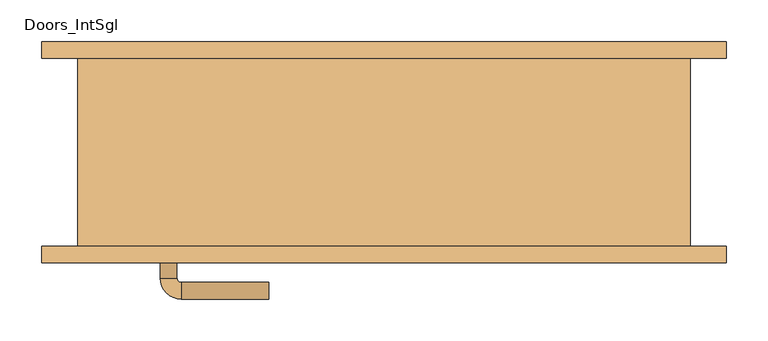
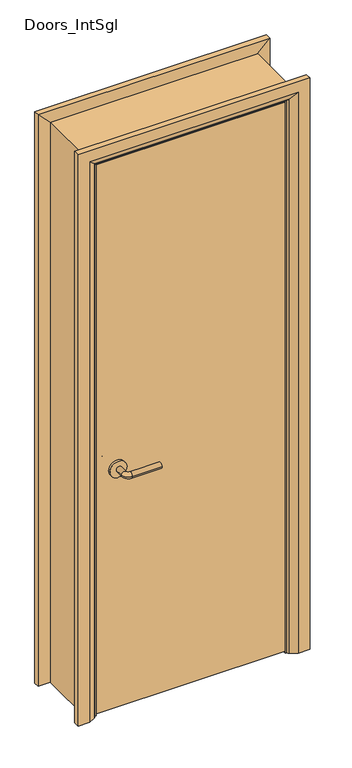
"""IFC4 building model written with IfcOpenShell, lengths in millimetres: door geometry, Doors_IntSgl."""

from ifc_helpers import new_model, si_unit, point, frame, frame_2d, origin, place, context, project, spatial, polyline, circle_curve, ellipse_curve, trimmed, segment, composite_curve, outline, extrude, faceted_brep, source, transform, mapped, element, save
from ifc_brep_helpers import plane_surface, cylinder_surface, revolved_surface, advanced_brep


def doors_intsgl_927b0b89(model_context):
    return source(origin(), model_context, "Body", "SolidModel", [
        advanced_brep(
        [(-268.0, -66.5, 900.0), (-248.0, -66.5, 900.0), (-268.0, -36.5, 900.0), (-248.0, -36.5, 900.0), (-243.0, -31.5, 900.0), (-243.0, -11.5, 900.0), (-138.0, -11.5, 900.0), (-138.0, -31.5, 900.0)],
        [
            (0, 1, circle_curve(frame((-258.0, -66.5, 900.0), z_axis=(0.0, -1.0, 0.0), x_axis=(1.0, 0.0, 0.0)), 10.0)),
            (1, 0, circle_curve(frame((-258.0, -66.5, 900.0), z_axis=(0.0, -1.0, 0.0), x_axis=(1.0, 0.0, 0.0)), 10.0)),
            (0, 2),
            (2, 3, circle_curve(frame((-258.0, -36.5, 900.0), z_axis=(0.0, -1.0, 0.0), x_axis=(1.0, 0.0, 0.0)), 10.0)),
            (3, 1),
            (3, 2, circle_curve(frame((-258.0, -36.5, 900.0), z_axis=(0.0, -1.0, 0.0), x_axis=(1.0, 0.0, 0.0)), 10.0)),
            (4, 3, circle_curve(frame((-243.0, -36.5, 900.0), z_axis=(0.0, 0.0, 1.0), x_axis=(-1.0, 0.0, 0.0)), 5.0)),
            (2, 5, circle_curve(frame((-243.0, -36.5, 900.0), z_axis=(0.0, 0.0, -1.0), x_axis=(-1.0, 0.0, 0.0)), 25.0)),
            (5, 4, circle_curve(frame((-243.0, -21.5, 900.0), z_axis=(-1.0, 0.0, 0.0), x_axis=(0.0, -1.0, 0.0)), 10.0)),
            (4, 5, circle_curve(frame((-243.0, -21.5, 900.0), z_axis=(-1.0, 0.0, 0.0), x_axis=(0.0, -1.0, 0.0)), 10.0)),
            (6, 7, circle_curve(frame((-138.0, -21.5, 900.0), z_axis=(1.0, 0.0, 0.0), x_axis=(0.0, -1.0, 0.0)), 10.0)),
            (7, 6, circle_curve(frame((-138.0, -21.5, 900.0), z_axis=(1.0, 0.0, 0.0), x_axis=(0.0, -1.0, 0.0)), 10.0)),
            (5, 6),
            (7, 4),
        ],
        [
            plane_surface(frame((-258.0, -66.5, 900.0), z_axis=(0.0, -1.0, 0.0), x_axis=(0.0, 0.0, 1.0))),
            cylinder_surface(frame((-258.0, -66.5, 900.0), z_axis=(0.0, -1.0, 0.0), x_axis=(1.0, 0.0, 0.0)), 10.0),
            revolved_surface(trimmed(ellipse_curve(frame((-258.0, -36.5, 900.0), z_axis=(0.0, -1.0, 0.0), x_axis=(1.0, 0.0, 0.0)), 10.0, 10.0), [point((-268.0, -36.5, 900.0))], [point((-248.0, -36.5, 900.0))], True, "CARTESIAN"), (-243.0, -36.5, 900.0), (0.0, 0.0, -1.0)),
            revolved_surface(trimmed(ellipse_curve(frame((-258.0, -36.5, 900.0), z_axis=(0.0, -1.0, 0.0), x_axis=(1.0, 0.0, 0.0)), 10.0, 10.0), [point((-248.0, -36.5, 900.0))], [point((-268.0, -36.5, 900.0))], True, "CARTESIAN"), (-243.0, -36.5, 900.0), (0.0, 0.0, -1.0)),
            plane_surface(frame((-138.0, -21.5, 900.0), z_axis=(1.0, 0.0, 0.0), x_axis=(0.0, 0.0, 1.0))),
            cylinder_surface(frame((-243.0, -21.5, 900.0), z_axis=(-1.0, 0.0, 0.0), x_axis=(0.0, -1.0, 0.0)), 10.0),
        ],
        [
            (0, [[1, 2]]),
            (1, [[-1, 3, 4, 5]]),
            (1, [[-2, -5, 6, -3]]),
            (2, [[7, -4, 8, 9]]),
            (3, [[-8, -6, -7, 10]]),
            (4, [[11, 12]]),
            (5, [[-9, 13, -12, 14]]),
            (5, [[-10, -14, -11, -13]]),
        ],
    ),
        extrude(outline(composite_curve([segment(trimmed(circle_curve(frame_2d((900.0, -260.5)), 30.0), [point((900.0, -290.5))], [point((900.0, -230.5))], False, "CARTESIAN"), True, "CONTINUOUS"), segment(trimmed(circle_curve(frame_2d((900.0, -260.5)), 30.0), [point((900.0, -230.5))], [point((900.0, -290.5))], False, "CARTESIAN"), True, "CONTINUOUS")], self_intersect=False)), frame((0.0, -74.5, 0.0), z_axis=(0.0, 1.0, 0.0), x_axis=(0.0, 0.0, 1.0)), (0.0, 0.0, 1.0), 8.0),
        advanced_brep(
        [(-268.0, -120.5, 900.0), (-248.0, -120.5, 900.0), (-248.0, -150.5, 900.0), (-268.0, -150.5, 900.0), (-243.0, -155.5, 900.0), (-243.0, -175.5, 900.0), (-138.0, -175.5, 900.0), (-138.0, -155.5, 900.0)],
        [
            (0, 1, circle_curve(frame((-258.0, -120.5, 900.0), z_axis=(0.0, 1.0, 0.0), x_axis=(1.0, 0.0, 0.0)), 10.0)),
            (1, 0, circle_curve(frame((-258.0, -120.5, 900.0), z_axis=(0.0, 1.0, 0.0), x_axis=(1.0, 0.0, 0.0)), 10.0)),
            (1, 2),
            (2, 3, circle_curve(frame((-258.0, -150.5, 900.0), z_axis=(0.0, 1.0, 0.0), x_axis=(1.0, 0.0, 0.0)), 10.0)),
            (3, 0),
            (3, 2, circle_curve(frame((-258.0, -150.5, 900.0), z_axis=(0.0, 1.0, 0.0), x_axis=(1.0, 0.0, 0.0)), 10.0)),
            (4, 5, circle_curve(frame((-243.0, -165.5, 900.0), z_axis=(-1.0, 0.0, 0.0), x_axis=(0.0, 1.0, 0.0)), 10.0)),
            (5, 3, circle_curve(frame((-243.0, -150.5, 900.0), z_axis=(0.0, 0.0, -1.0), x_axis=(-1.0, 0.0, 0.0)), 25.0)),
            (2, 4, circle_curve(frame((-243.0, -150.5, 900.0), z_axis=(0.0, 0.0, 1.0), x_axis=(-1.0, 0.0, 0.0)), 5.0)),
            (5, 4, circle_curve(frame((-243.0, -165.5, 900.0), z_axis=(-1.0, 0.0, 0.0), x_axis=(0.0, 1.0, 0.0)), 10.0)),
            (6, 7, circle_curve(frame((-138.0, -165.5, 900.0), z_axis=(1.0, 0.0, 0.0), x_axis=(0.0, 1.0, 0.0)), 10.0)),
            (7, 6, circle_curve(frame((-138.0, -165.5, 900.0), z_axis=(1.0, 0.0, 0.0), x_axis=(0.0, 1.0, 0.0)), 10.0)),
            (4, 7),
            (6, 5),
        ],
        [
            plane_surface(frame((-258.0, -120.5, 900.0), z_axis=(0.0, 1.0, 0.0), x_axis=(0.0, 0.0, 1.0))),
            cylinder_surface(frame((-258.0, -120.5, 900.0), z_axis=(0.0, 1.0, 0.0), x_axis=(1.0, 0.0, 0.0)), 10.0),
            revolved_surface(trimmed(ellipse_curve(frame((-258.0, -150.5, 900.0), z_axis=(0.0, -1.0, 0.0), x_axis=(1.0, 0.0, 0.0)), 10.0, 10.0), [point((-268.0, -150.5, 900.0))], [point((-248.0, -150.5, 900.0))], True, "CARTESIAN"), (-243.0, -150.5, 900.0), (0.0, 0.0, -1.0)),
            revolved_surface(trimmed(ellipse_curve(frame((-258.0, -150.5, 900.0), z_axis=(0.0, -1.0, 0.0), x_axis=(1.0, 0.0, 0.0)), 10.0, 10.0), [point((-248.0, -150.5, 900.0))], [point((-268.0, -150.5, 900.0))], True, "CARTESIAN"), (-243.0, -150.5, 900.0), (0.0, 0.0, -1.0)),
            plane_surface(frame((-138.0, -165.5, 900.0), z_axis=(1.0, 0.0, 0.0), x_axis=(0.0, 0.0, 1.0))),
            cylinder_surface(frame((-243.0, -165.5, 900.0), z_axis=(-1.0, 0.0, 0.0), x_axis=(0.0, 1.0, 0.0)), 10.0),
        ],
        [
            (0, [[1, 2]]),
            (1, [[3, 4, 5, -2]]),
            (1, [[-5, 6, -3, -1]]),
            (2, [[7, 8, -4, 9]]),
            (3, [[10, -9, -6, -8]]),
            (4, [[11, 12]]),
            (5, [[13, -11, 14, -7]]),
            (5, [[-14, -12, -13, -10]]),
        ],
    ),
        extrude(outline(composite_curve([segment(trimmed(circle_curve(frame_2d((900.0, -260.5)), 30.0), [point((900.0, -290.5))], [point((900.0, -230.5))], False, "CARTESIAN"), True, "CONTINUOUS"), segment(trimmed(circle_curve(frame_2d((900.0, -260.5)), 30.0), [point((900.0, -230.5))], [point((900.0, -290.5))], False, "CARTESIAN"), True, "CONTINUOUS")], self_intersect=False)), frame((0.0, -120.5, 0.0), z_axis=(0.0, 1.0, 0.0), x_axis=(0.0, 0.0, 1.0)), (0.0, 0.0, 1.0), 8.0),
        extrude(outline(polyline([(333.0, -74.5), (333.0, -112.5), (-333.0, -112.5), (-333.0, -74.5), (333.0, -74.5)])), frame((0.0, 0.0, 8.0), z_axis=(0.0, 0.0, 1.0), x_axis=(1.0, 0.0, 0.0)), (0.0, 0.0, 1.0), 2050.0),
        faceted_brep([(-335.0, -112.5, 0.0), (-367.0, -112.5, 0.0), (-367.0, 112.5, 0.0), (-335.0, 112.5, 0.0), (-335.0, 112.5, 2060.0), (-335.0, -112.5, 2060.0), (-367.0, 112.5, 2092.0), (-367.0, -112.5, 2092.0), (335.0, -112.5, 0.0), (335.0, 112.5, 0.0), (367.0, 112.5, 0.0), (367.0, -112.5, 0.0), (335.0, -112.5, 2060.0), (367.0, -112.5, 2092.0), (367.0, 112.5, 2092.0), (335.0, 112.5, 2060.0)], [[[0, 1, 2, 3]], [[3, 4, 5, 0]], [[2, 6, 4, 3]], [[1, 7, 6, 2]], [[0, 5, 7, 1]], [[8, 9, 10, 11]], [[12, 8, 11, 13]], [[13, 11, 10, 14]], [[14, 10, 9, 15]], [[15, 9, 8, 12]], [[4, 15, 12, 5]], [[6, 14, 15, 4]], [[7, 13, 14, 6]], [[5, 12, 13, 7]]]),
        advanced_brep(
        [(-410.0, 132.5, 0.0), (-370.0, 132.5, 0.0), (-344.0, 118.5, 0.0), (-340.0, 112.5, 0.0), (-410.0, 112.5, 0.0), (-410.0, 112.5, 2135.0), (-410.0, 132.5, 2135.0), (-340.0, 112.5, 2065.0), (-344.0, 118.5, 2069.0), (-370.0, 132.5, 2095.0), (410.0, 132.5, 0.0), (410.0, 112.5, 0.0), (340.0, 112.5, 0.0), (344.0, 118.5, 0.0), (370.0, 132.5, 0.0), (410.0, 132.5, 2135.0), (370.0, 132.5, 2095.0), (344.0, 118.5, 2069.0), (340.0, 112.5, 2065.0), (410.0, 112.5, 2135.0)],
        [
            (0, 1),
            (1, 2),
            (2, 3, circle_curve(frame((-348.0, 111.5, 0.0), z_axis=(0.0, 0.0, -1.0), x_axis=(-1.0, 0.0, 0.0)), 8.0622577)),
            (3, 4),
            (4, 0),
            (4, 5),
            (5, 6),
            (6, 0),
            (3, 7),
            (7, 5),
            (2, 8),
            (8, 7, ellipse_curve(frame((-348.0, 111.5, 2073.0), z_axis=(-0.7071067811865475, 0.0, -0.7071067811865475), x_axis=(0.7071067811865474, 0.0, -0.7071067811865476)), 11.4017543, 8.0622577)),
            (1, 9),
            (9, 8),
            (6, 9),
            (10, 11),
            (11, 12),
            (12, 13, circle_curve(frame((348.0, 111.5, 0.0), z_axis=(0.0, 0.0, -1.0), x_axis=(1.0, 0.0, 0.0)), 8.0622577)),
            (13, 14),
            (14, 10),
            (15, 10),
            (14, 16),
            (16, 15),
            (13, 17),
            (17, 16),
            (12, 18),
            (18, 17, ellipse_curve(frame((348.0, 111.5, 2073.0), z_axis=(0.7071067811865475, 0.0, -0.7071067811865475), x_axis=(0.7071067811865474, 0.0, 0.7071067811865476)), 11.4017543, 8.0622577)),
            (11, 19),
            (19, 18),
            (15, 19),
            (5, 19),
            (15, 6),
            (7, 18),
            (8, 17),
            (9, 16),
        ],
        [
            plane_surface(frame((-340.0, 185.3010989, 0.0), z_axis=(0.0, 0.0, -1.0), x_axis=(1.0, 0.0, 0.0))),
            plane_surface(frame((-410.0, 132.5, 0.0), z_axis=(-1.0, 0.0, 0.0), x_axis=(0.0, 0.0, 1.0))),
            plane_surface(frame((-410.0, 112.5, 0.0), z_axis=(0.0, -1.0, 0.0), x_axis=(0.0, 0.0, 1.0))),
            cylinder_surface(frame((-348.0, 111.5, 0.0), z_axis=(0.0, 0.0, -1.0), x_axis=(-1.0, 0.0, 0.0)), 8.0622577),
            plane_surface(frame((-344.0, 118.5, 0.0), z_axis=(0.4740998230350183, 0.8804710999221749, 0.0), x_axis=(0.0, 0.0, 1.0))),
            plane_surface(frame((-370.0, 132.5, 0.0), z_axis=(0.0, 1.0, 0.0), x_axis=(0.0, 0.0, 1.0))),
            plane_surface(frame((340.0, 185.3010989, 0.0), z_axis=(0.0, 0.0, -1.0), x_axis=(-1.0, 0.0, 0.0))),
            plane_surface(frame((370.0, 132.5, 2095.0), z_axis=(0.0, 1.0, 0.0), x_axis=(0.0, 0.0, -1.0))),
            plane_surface(frame((344.0, 118.5, 2069.0), z_axis=(-0.4740998230350183, 0.8804710999221749, 0.0), x_axis=(0.0, 0.0, -1.0))),
            cylinder_surface(frame((348.0, 111.5, 2065.0), z_axis=(0.0, 0.0, 1.0), x_axis=(1.0, 0.0, 0.0)), 8.0622577),
            plane_surface(frame((410.0, 112.5, 2135.0), z_axis=(0.0, -1.0, 0.0), x_axis=(0.0, 0.0, -1.0))),
            plane_surface(frame((410.0, 132.5, 2135.0), z_axis=(1.0, 0.0, 0.0), x_axis=(0.0, 0.0, -1.0))),
            plane_surface(frame((-410.0, 132.5, 2135.0), z_axis=(0.0, 0.0, 1.0), x_axis=(1.0, 0.0, 0.0))),
            plane_surface(frame((-410.0, 112.5, 2135.0), z_axis=(0.0, -1.0, 0.0), x_axis=(1.0, 0.0, 0.0))),
            cylinder_surface(frame((-340.0, 111.5, 2073.0), z_axis=(-1.0, 0.0, 0.0), x_axis=(0.0, 0.0, 1.0)), 8.0622577),
            plane_surface(frame((-344.0, 118.5, 2069.0), z_axis=(0.0, 0.8804710999221749, -0.4740998230350183), x_axis=(1.0, 0.0, 0.0))),
            plane_surface(frame((-370.0, 132.5, 2095.0), z_axis=(0.0, 1.0, 0.0), x_axis=(1.0, 0.0, 0.0))),
        ],
        [
            (0, [[1, 2, 3, 4, 5]]),
            (1, [[6, 7, 8, -5]]),
            (2, [[9, 10, -6, -4]]),
            (3, [[11, 12, -9, -3]]),
            (4, [[13, 14, -11, -2]]),
            (5, [[-8, 15, -13, -1]]),
            (6, [[16, 17, 18, 19, 20]]),
            (7, [[21, -20, 22, 23]]),
            (8, [[-22, -19, 24, 25]]),
            (9, [[-24, -18, 26, 27]]),
            (10, [[-26, -17, 28, 29]]),
            (11, [[-28, -16, -21, 30]]),
            (12, [[31, -30, 32, -7]]),
            (13, [[33, -29, -31, -10]]),
            (14, [[34, -27, -33, -12]]),
            (15, [[35, -25, -34, -14]]),
            (16, [[-32, -23, -35, -15]]),
        ],
    ),
        extrude(outline(polyline([(0.0, -316.0), (2041.0, -316.0), (2041.0, 316.0), (0.0, 316.0), (0.0, 335.0), (2060.0, 335.0), (2060.0, -335.0), (0.0, -335.0), (0.0, -316.0)])), frame((0.0, -72.5, 0.0), z_axis=(0.0, 1.0, 0.0), x_axis=(0.0, 0.0, 1.0)), (0.0, 0.0, 1.0), 32.0),
        advanced_brep(
        [(410.0, -132.5, 0.0), (370.0, -132.5, 0.0), (344.0, -118.5, 0.0), (340.0, -112.5, 0.0), (410.0, -112.5, 0.0), (410.0, -112.5, 2135.0), (410.0, -132.5, 2135.0), (340.0, -112.5, 2065.0), (-340.0, -112.5, 2065.0), (-340.0, -112.5, 0.0), (-410.0, -112.5, 0.0), (-410.0, -112.5, 2135.0), (344.0, -118.5, 2069.0), (370.0, -132.5, 2095.0), (-410.0, -132.5, 2135.0), (-410.0, -132.5, 0.0), (-370.0, -132.5, 0.0), (-370.0, -132.5, 2095.0), (-344.0, -118.5, 0.0), (-344.0, -118.5, 2069.0)],
        [
            (0, 1),
            (1, 2),
            (2, 3, circle_curve(frame((348.0, -111.5, 0.0), z_axis=(0.0, 0.0, -1.0), x_axis=(1.0, 0.0, 0.0)), 8.0622577)),
            (3, 4),
            (4, 0),
            (4, 5),
            (5, 6),
            (6, 0),
            (3, 7),
            (7, 8),
            (8, 9),
            (9, 10),
            (10, 11),
            (11, 5),
            (2, 12),
            (12, 7, ellipse_curve(frame((348.0, -111.5, 2073.0), z_axis=(0.7071067811865475, 0.0, -0.7071067811865475), x_axis=(-0.7071067811865474, 0.0, -0.7071067811865476)), 11.4017543, 8.0622577)),
            (1, 13),
            (13, 12),
            (6, 14),
            (14, 15),
            (15, 16),
            (16, 17),
            (17, 13),
            (10, 15),
            (14, 11),
            (9, 18, circle_curve(frame((-348.0, -111.5, 0.0), z_axis=(0.0, 0.0, -1.0), x_axis=(-1.0, 0.0, 0.0)), 8.0622577)),
            (18, 16),
            (19, 18),
            (8, 19, ellipse_curve(frame((-348.0, -111.5, 2073.0), z_axis=(-0.7071067811865475, 0.0, -0.7071067811865475), x_axis=(-0.7071067811865474, 0.0, 0.7071067811865476)), 11.4017543, 8.0622577)),
            (19, 17),
            (12, 19),
        ],
        [
            plane_surface(frame((340.0, -112.5, 0.0), z_axis=(0.0, 0.0, -1.0), x_axis=(0.0, 1.0, 0.0))),
            plane_surface(frame((410.0, -132.5, 0.0), z_axis=(1.0, 0.0, 0.0), x_axis=(0.0, 0.0, 1.0))),
            plane_surface(frame((410.0, -112.5, 0.0), z_axis=(0.0, 1.0, 0.0), x_axis=(0.0, 0.0, 1.0))),
            cylinder_surface(frame((348.0, -111.5, 0.0), z_axis=(0.0, 0.0, -1.0), x_axis=(1.0, 0.0, 0.0)), 8.0622577),
            plane_surface(frame((344.0, -118.5, 0.0), z_axis=(-0.4740998230350126, -0.880471099922178, 0.0), x_axis=(0.0, 0.0, 1.0))),
            plane_surface(frame((370.0, -132.5, 0.0), z_axis=(0.0, -1.0, 0.0), x_axis=(0.0, 0.0, 1.0))),
            plane_surface(frame((-410.0, -132.5, 2135.0), z_axis=(-1.0, 0.0, 0.0), x_axis=(0.0, 0.0, -1.0))),
            plane_surface(frame((-340.0, -112.5, 0.0), z_axis=(0.0, 0.0, -1.0), x_axis=(0.0, 1.0, 0.0))),
            cylinder_surface(frame((-348.0, -111.5, 2065.0), z_axis=(0.0, 0.0, 1.0), x_axis=(-1.0, 0.0, 0.0)), 8.0622577),
            plane_surface(frame((-344.0, -118.5, 2069.0), z_axis=(0.47409982303501824, -0.8804710999221749, 0.0), x_axis=(0.0, 0.0, -1.0))),
            plane_surface(frame((410.0, -132.5, 2135.0), z_axis=(0.0, 0.0, 1.0), x_axis=(-1.0, 0.0, 0.0))),
            cylinder_surface(frame((340.0, -111.5, 2073.0), z_axis=(1.0, 0.0, 0.0), x_axis=(0.0, 0.0, 1.0)), 8.0622577),
            plane_surface(frame((344.0, -118.5, 2069.0), z_axis=(0.0, -0.8804710999221764, -0.4740998230350154), x_axis=(-1.0, 0.0, 0.0))),
        ],
        [
            (0, [[1, 2, 3, 4, 5]]),
            (1, [[6, 7, 8, -5]]),
            (2, [[9, 10, 11, 12, 13, 14, -6, -4]]),
            (3, [[15, 16, -9, -3]]),
            (4, [[17, 18, -15, -2]]),
            (5, [[-8, 19, 20, 21, 22, 23, -17, -1]]),
            (6, [[-13, 24, -20, 25]]),
            (7, [[-24, -12, 26, 27, -21]]),
            (8, [[28, -26, -11, 29]]),
            (9, [[-22, -27, -28, 30]]),
            (10, [[-14, -25, -19, -7]]),
            (11, [[31, -29, -10, -16]]),
            (12, [[-23, -30, -31, -18]]),
        ],
    ),
    ])


if __name__ == "__main__":
    model = new_model("IFC4")
    model_context = context("Model", 3, world=origin())
    ifc_project = project(units=[si_unit("LENGTHUNIT", "METRE", prefix="MILLI")], contexts=[model_context])
    site = spatial("IfcSite", under=ifc_project)
    building = spatial("IfcBuilding", under=site)
    placement = place(None, origin())
    doors_intsgl_shape = doors_intsgl_927b0b89(model_context)
    element("IfcDoor", 1, ObjectType="Doors_IntSgl", at=placement, inside=building, context=model_context, shape_type="MappedRepresentation", body=[
        mapped(doors_intsgl_shape, transform((0.0, 0.0, 0.0), x_axis=(1.0, 0.0, 0.0), y_axis=(0.0, 1.0, 0.0), z_axis=(0.0, 0.0, 1.0))),
    ])
    save(model, "model.ifc")

# Revit data of these elements
# Type "Doors_IntSgl"
#   Type Mark = "45"
#   Type Comments = "Internal Single"
#   Operation = "SingleSwingRight"
#   Manufacturer = "Revit"
#   Keynote = "L20"
#   Description = "Internal Single Door"
#   Analytic Construction = "Metal"
#   UnderCut = 8 mm
#   Tolerance = 2 mm
#   Thickness = 38 mm
#   Thermal Resistance (R) = 0.270117 (m²·K)/W
#   Structural Tolerance = 8 mm
#   StopDepth = 32 mm
#   Stop Thickness = 19 mm
#   Rough Width = 750 mm
#   Rough Height = 2100 mm
#   Height to Top Lock Rail = 1000 mm
#   Heat Transfer Coefficient (U) = 3.7021 W/(m²·K)
#   Handle Z Distance = 900 mm
#   Handle X Distance = 75 mm
#   Frame Thickness = 32 mm
#   Door Panel Width = 666 mm
#   Door Panel Thickness = 38 mm
#   Door Panel Offset = 0 mm
#   Height = 2100 mm
#   Width = 750 mm
#   Door Panel Height = 2050 mm
#   Architrave Setback = 5 mm
#   Vis - Ironmongery = yes
#   Define Thermal Properties by = 1
#   Material Ironmongery = Door - Handle
#   Material Frame = Door - Frame/Mullion (1)
#   Material Door = Door - Panel
#   Material Architrave = Door - Architrave
#   Visual Light Transmittance = 0
#   Solar Heat Gain Coefficient = 0
#   Function = (empty or 0)
#   Wall Closure = (empty or 0)
# Element 1 (IfcDoor, "Doors_IntSgl")
#   Materials on its faces: "Door - Architrave", "Door - Handle", "Door - Frame/Mullion (1)", "Door - Panel"
# Materials
#   "Door - Handle": colour RGB 0 0 0, transparency 0, Cost = 0
#   "Door - Frame/Mullion (1)": class "Wood", colour RGB 212 179 113, transparency 0, Keynote = "L20", Cost = 0
#   "Door - Panel": class "Wood", colour RGB 210 159 95, transparency 0, Cost = 0
#   "Door - Architrave": class "Wood", colour RGB 154 90 5, transparency 0, Keynote = "P20", Cost = 0
